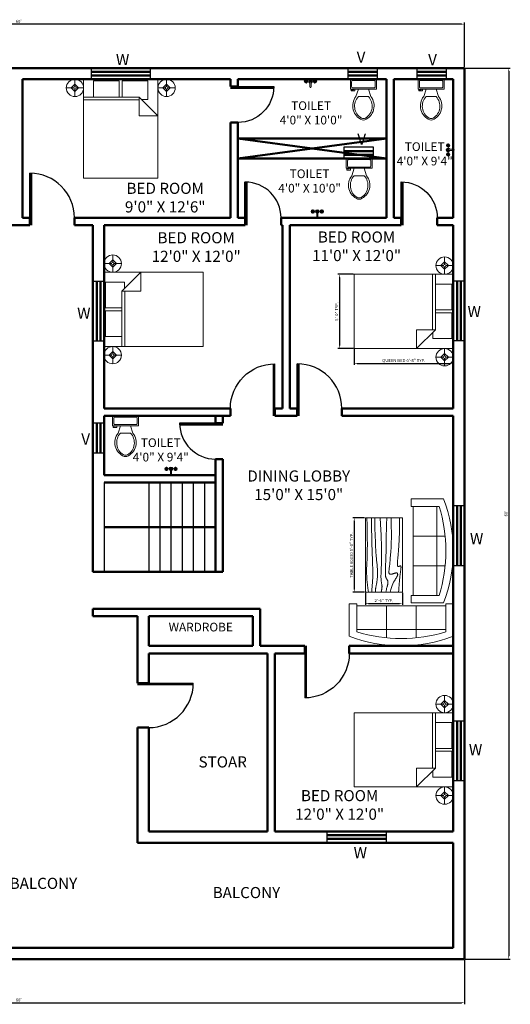
# Model space of a CAD drawing. Units: inches. Extents: x 2663 to 4539, y 2314 to 3111.
# Tile 4 of 4: x 4143 to 4539, y 2316 to 3111. Entities that reach past the tile are written whole.
import ezdxf

# ---------------------------------------------------------------- set-up
doc = ezdxf.new("R2010")
doc.units = ezdxf.units.IN
for name, color, linetype, lineweight in [('A-ANNO-DIMS', 2, 'Continuous', 18), ('A-ANNO-TEXT', 7, 'Continuous', 18), ('A-AREA-IDEN', 3, 'Continuous', 25), ('A-DOOR', 4, 'Continuous', 25), ('A-FLOR-FIXT', 8, 'Continuous', 18), ('A-FLOR-STRS', 2, 'Continuous', 25), ('A-FURN', 8, 'Continuous', 18), ('A-GLAZ', 3, 'Continuous', 25), ('A-WALL', 7, 'Continuous', 50)]:
    doc.layers.add(name, color=color, linetype=linetype, lineweight=lineweight)
doc.styles.get("Standard").update_dxf_attribs({"font": 'arial.ttf'})
doc.dimstyles.new('ISO-25', dxfattribs={"dimtxt": 2.5, "dimasz": 2.5, "dimexe": 1.25, "dimexo": 0.625, "dimtad": 1, "dimdec": 0, "dimlunit": 3, "dimtxsty": 'Standard', "dimcen": 2.5, "dimadec": 0, "dimazin": 0, "dimtfac": 1, "dimtdec": 0, "dimtmove": 0, "dimatfit": 3, "dimfxl": 1, "dimarcsym": 0})

# ---------------------------------------------------------------- blocks, each defined once
blk = doc.blocks.new('Toilet - top')
for p, q in [((9.5, -6), (9.5, -2)), ((-10, -8.5), (-8, -8.5)), ((-10, -9.5), (-10, -8.5)), ((-7, -9.5), (-10, -9.5)), ((-8, -8.5), (-8, -8)), ((-7, -8), (-7, -9.5)), ((-4, -8), (-6, -14)), ((4, -14), (-4, -14)), ((4, -8), (6, -14))]:
    blk.add_line(p, q)
blk.add_lwpolyline([(10.5, -8), (10.5, 0), (-10.5, 0), (-10.5, -8)], close=True)
for points in [[(-9.5, -2), (-9.5, -6)], [(8.5, -1), (-8.5, -1)], [(-8.5, -7), (8.5, -7)]]:
    blk.add_lwpolyline(points)
for centre, radius, start, end in [((-8.62, -1.88), 0.884, 81.8699, 188.1301), ((-8.62, -6.12), 0.884, 171.8699, 278.1301), ((8.62, -1.88), 0.884, 351.8699, 98.1301), ((8.62, -6.12), 0.884, 261.8699, 8.1301), ((3.52, -21.58), 12.17, 141.46911, 247.97143), ((4.2, -21.82), 11.33, 136.36773, 238.94682), ((-3.52, -21.58), 12.17, 292.02843, 38.53071), ((-4.2, -21.82), 11.33, 301.05301, 43.63209), ((0, -27.88), 4, 245.73182, 294.26817), ((0, -29), 4, 254.86053, 285.13947)]:
    blk.add_arc(centre, radius, start, end)
blk = doc.blocks.new('Faucet - Bathroom top')
for p, q in [((-4.107, 0.125), (-4.375, 0.125)), ((-3.75, 0.4788), (-3.75, 0.75)), ((-3.5, 0.482), (-3.5, 0.75)), ((-3.1461, 0.125), (-2.875, 0.125)), ((3.143, 0.125), (2.875, 0.125)), ((3.5, 0.4788), (3.5, 0.75)), ((3.75, 0.482), (3.75, 0.75)), ((4.1039, 0.125), (4.375, 0.125)), ((-4.1039, -0.125), (-4.375, -0.125)), ((-3.75, -0.4821), (-3.75, -0.75)), ((-3.5, -0.4789), (-3.5, -0.75)), ((-3.143, -0.125), (-2.875, -0.125)), ((-0.5, -0.8639), (-0.5, -4.5)), ((0.5, -4.5), (0.5, -0.8631)), ((3.1461, -0.125), (2.875, -0.125)), ((3.5, -0.4821), (3.5, -0.75)), ((3.75, -0.4789), (3.75, -0.75)), ((4.107, -0.125), (4.375, -0.125))]:
    blk.add_line(p, q)
for centre, radius in [((-3.625, 0), 1.375), ((-4.625, 0), 0.2795), ((-3.625, 0), 0.5), ((-3.625, 1), 0.2795), ((-2.625, 0), 0.2795), ((0, 0), 0.5), ((3.625, 0), 1.375), ((2.625, 0), 0.2795), ((3.625, 0), 0.5), ((3.625, 1), 0.2795), ((4.625, 0), 0.2795), ((-3.625, -1), 0.2795), ((3.625, -1), 0.2795)]:
    blk.add_circle(centre, radius)
for centre, radius, start, end in [((-3.625, 0), 1, 105.2407, 164.2093), ((-3.625, 0), 1, 16.44125, 74.07887), ((0, 0), 1.5, 289.6514, 250.3603), ((0, 0), 1, 300.3431, 239.7554), ((3.625, 0), 1, 106.12, 164.0884), ((3.625, 0), 1, 16.23422, 73.90469), ((-3.625, 0), 1, 196.2342, 253.9047), ((-3.625, 0), 1, 286.12, 344.0884), ((0, -4.5), 0.5, 180, 0), ((3.625, 0), 1, 196.4413, 254.0789), ((3.625, 0), 1, 285.2407, 344.2093)]:
    blk.add_arc(centre, radius, start, end)
blk = doc.blocks.new('Bed - Queen')
for p, q in [((0, -80.00003), (0, 0)), ((0, 0), (59.99999, 0)), ((59.99999, 0), (59.99999, -80.00003)), ((7.99999, -1.2), (28.79998, -1.2)), ((7.99999, -14.4), (7.99999, -1.2)), ((28.79998, -1.2), (28.79998, -14.4)), ((31.19999, -1.2), (51.99999, -1.2)), ((31.19999, -14.4), (31.19999, -1.2)), ((51.99999, -1.2), (51.99999, -16.4)), ((0, -14.4), (44.8, -14.4)), ((59.99999, -29.6), (44.8, -14.4)), ((44.8, -14.4), (44.8, -29.6)), ((44.8, -16.8), (0, -16.8)), ((51.99999, -16.4), (46.79936, -16.4)), ((44.8, -29.6), (59.99999, -29.6)), ((59.99999, -80.00003), (0, -80.00003))]:
    blk.add_line(p, q)
blk = doc.blocks.new('Lamp - Table')
for p, q in [((-1, 0), (-7, 0)), ((0, 3), (-3, 0)), ((-3, 0), (0, -3)), ((0, 7), (0, 1)), ((3, 0), (0, 3)), ((0, -3), (3, 0)), ((1, 0), (7, 0)), ((0, -1), (0, -7))]:
    blk.add_line(p, q)
for radius in [7, 1]:
    blk.add_circle((0, 0), radius)
blk = doc.blocks.new('Sofa - Roundback 7 ft.')
for p, q in [((-12.00002, -32.4421), (-12.00003, -6.5971)), ((11.99997, -32.4421), (11.99998, -6.5971)), ((-36.000027, -34), (-36.000027, -11.4696)), ((-35.999844, -13.3819), (35.9998, -13.3819)), ((35.99998, -34), (35.99998, -11.4696)), ((-36.000027, -32.4421), (35.99998, -32.4421))]:
    blk.add_line(p, q)
for points in [[(-36.000027, -34), (-42.000027, -34), (-42.000027, -8)], [(41.99998, -8), (41.99998, -34), (35.99998, -34)]]:
    blk.add_lwpolyline(points)
for centre, radius, start, end in [((0, -114.25), 114.25, 68.43141, 111.5686), ((-0.00001, -127.1968), 121.1968, 72.72033, 107.2797)]:
    blk.add_arc(centre, radius, start, end)
blk = doc.blocks.new('Table - Rectangular Woodgrain 60 x 30 in.')
for p, q in [((0, 0), (0, -30)), ((60, 0), (0, 0)), ((60, -30), (60, 0)), ((0, -30), (60, -30))]:
    blk.add_line(p, q)
for points in [[(0, -2.4), (4.8155, -2.418), (9.0302, -2.4688), (12.709, -2.5477), (15.9167, -2.65), (18.7181, -2.7711), (21.1781, -2.9063), (23.3616, -3.0508), (25.3333, -3.2), (27.1477, -3.3495), (28.8172, -3.4958), (30.3437, -3.636), (31.7291, -3.7667), (32.9756, -3.8849), (34.0849, -3.9875), (35.059, -4.0714), (35.9, -4.1334), (36.6114, -4.1711), (37.2041, -4.1854), (37.6906, -4.1779), (38.0833, -4.15), (38.3948, -4.1034), (38.6375, -4.0396), (38.8239, -3.9602), (38.9666, -3.8667), (39.0764, -3.7608), (39.1573, -3.6448), (39.2116, -3.521), (39.2416, -3.3917), (39.2498, -3.2593), (39.2385, -3.1261), (39.21, -2.9944), (39.1666, -2.8667), (39.111, -2.7447), (39.0468, -2.6281), (38.978, -2.5163), (38.9083, -2.4083), (38.8418, -2.3035), (38.7823, -2.201), (38.7337, -2.1001), (38.7, -2), (38.6844, -1.9003), (38.6875, -1.8021), (38.7094, -1.707), (38.75, -1.6167), (38.8094, -1.5326), (38.8875, -1.4563), (38.9844, -1.3893), (39.1, -1.3333), (39.2351, -1.2896), (39.3937, -1.2583), (39.5804, -1.2396), (39.8, -1.2333), (40.057, -1.2396), (40.3562, -1.2583), (40.7023, -1.2896), (41.1, -1.3333), (41.5547, -1.3895), (42.0755, -1.4573), (42.6721, -1.5361), (43.3542, -1.625), (44.1316, -1.7233), (45.014, -1.8302), (46.0114, -1.9449), (47.1333, -2.0667), (48.3862, -2.1947), (49.7625, -2.3281), (51.2513, -2.4663), (52.8416, -2.6083), (54.5226, -2.7535), (56.2833, -2.9011), (58.1127, -3.0501), (60, -3.2)], [(0, -9.2), (6.5759, -9.0858), (11.9385, -9.0365), (16.2527, -9.0418), (19.6833, -9.0917), (22.3952, -9.1759), (24.5531, -9.2844), (26.322, -9.4069), (27.8666, -9.5333), (29.3241, -9.6553), (30.7203, -9.7719), (32.0532, -9.8837), (33.3208, -9.9917), (34.5213, -10.0965), (35.6526, -10.199), (36.7128, -10.2999), (37.7, -10.4), (38.6129, -10.4996), (39.4531, -10.5969), (40.223, -10.6895), (40.925, -10.775), (41.5613, -10.8512), (42.1344, -10.9156), (42.6465, -10.966), (43.1, -11), (43.4976, -11.0158), (43.8437, -11.0136), (44.143, -10.9942), (44.4, -10.9583), (44.6195, -10.9069), (44.8062, -10.8406), (44.9648, -10.7603), (45.1, -10.6667), (45.2155, -10.5598), (45.3114, -10.4365), (45.3871, -10.2929), (45.4416, -10.125), (45.4743, -9.929), (45.4844, -9.7011), (45.4709, -9.4371), (45.4333, -9.1333), (45.3716, -8.7883), (45.2896, -8.4104), (45.1919, -8.0107), (45.0833, -7.6), (44.9685, -7.1893), (44.8521, -6.7896), (44.7388, -6.4117), (44.6333, -6.0667), (44.54, -5.7628), (44.4614, -5.4979), (44.4001, -5.2675), (44.3583, -5.0667), (44.3384, -4.8909), (44.3427, -4.7354), (44.3736, -4.5956), (44.4333, -4.4667), (44.5236, -4.3453), (44.6427, -4.2333), (44.7884, -4.1339), (44.9583, -4.05), (45.1501, -3.9849), (45.3614, -3.9417), (45.59, -3.9234), (45.8333, -3.9333), (46.0915, -3.9749), (46.3734, -4.0531), (46.6906, -4.1736), (47.0542, -4.3417), (47.4756, -4.5629), (47.9661, -4.8427), (48.5372, -5.1866), (49.2, -5.6), (49.9676, -6.0844), (50.8594, -6.625), (51.8965, -7.2031), (53.1, -7.8), (54.491, -8.3969), (56.0906, -8.975), (57.9199, -9.5156), (60, -10)], [(0, -12.8), (5.1847, -12.9322), (9.6213, -13.0323), (13.3963, -13.1059), (16.5958, -13.1583), (19.3063, -13.1952), (21.614, -13.2219), (23.6054, -13.2439), (25.3666, -13.2667), (26.9728, -13.2947), (28.4531, -13.3281), (29.8256, -13.3663), (31.1083, -13.4083), (32.3191, -13.4535), (33.476, -13.501), (34.597, -13.5501), (35.7, -13.6), (36.7984, -13.6497), (37.8875, -13.6979), (38.9578, -13.743), (40, -13.7833), (41.0047, -13.8174), (41.9625, -13.8438), (42.864, -13.8607), (43.7, -13.8667), (44.4631, -13.8604), (45.1552, -13.8417), (45.7801, -13.8104), (46.3416, -13.7667), (46.8439, -13.7104), (47.2906, -13.6417), (47.6858, -13.5604), (48.0333, -13.4667), (48.3375, -13.3608), (48.6042, -13.2448), (48.8396, -13.121), (49.05, -12.9917), (49.2417, -12.8593), (49.4208, -12.7261), (49.5937, -12.5944), (49.7667, -12.4667), (49.9452, -12.3451), (50.1323, -12.2313), (50.3303, -12.1268), (50.5416, -12.0333), (50.7686, -11.9524), (51.0135, -11.8854), (51.2788, -11.8341), (51.5666, -11.8), (51.8785, -11.7843), (52.2116, -11.7865), (52.562, -11.8059), (52.926, -11.8417), (53.2998, -11.8931), (53.6795, -11.9594), (54.0614, -12.0397), (54.4416, -12.1333), (54.8223, -12.2401), (55.2293, -12.3625), (55.6942, -12.5037), (56.2489, -12.6667), (56.9251, -12.8547), (57.7545, -13.0708), (58.7689, -13.3182), (60, -13.6)], [(0, -18), (5.124, -17.7273), (9.6609, -17.5057), (13.6705, -17.3303), (17.2125, -17.1958), (20.3467, -17.0973), (23.1328, -17.0297), (25.6307, -16.9878), (27.9, -16.9667), (29.9928, -16.9617), (31.9302, -16.9703), (33.7254, -16.9907), (35.3917, -17.0208), (36.9423, -17.0588), (38.3906, -17.1026), (39.7499, -17.1503), (41.0333, -17.2), (42.2519, -17.2496), (43.4073, -17.2969), (44.4986, -17.3395), (45.525, -17.375), (46.4858, -17.4012), (47.3802, -17.4156), (48.2074, -17.416), (48.9667, -17.4), (49.6583, -17.3662), (50.2872, -17.3167), (50.8595, -17.2547), (51.3812, -17.1833), (51.8584, -17.1057), (52.2971, -17.025), (52.7034, -16.9443), (53.0833, -16.8667), (53.443, -16.7951), (53.789, -16.7313), (54.128, -16.6768), (54.4666, -16.6334), (54.8115, -16.6024), (55.1693, -16.5854), (55.5465, -16.5841), (55.95, -16.6), (56.3828, -16.6337), (56.8346, -16.6823), (57.2915, -16.7418), (57.7396, -16.8084), (58.165, -16.878), (58.5539, -16.9469), (58.8924, -17.0111), (59.1666, -17.0667), (59.3679, -17.1107), (59.5078, -17.1438), (59.6032, -17.1675), (59.6708, -17.1833), (59.7275, -17.193), (59.7901, -17.1979), (59.8753, -17.1998), (60, -17.2)], [(0, -22.4), (8.0098, -22.2501), (14.4094, -22.1011), (19.4168, -21.9535), (23.25, -21.8083), (26.1269, -21.6663), (28.2656, -21.5281), (29.884, -21.3947), (31.2, -21.2667), (32.3967, -21.1448), (33.5172, -21.0292), (34.5697, -20.9198), (35.5625, -20.8167), (36.5037, -20.7198), (37.4015, -20.6292), (38.2642, -20.5448), (39.1, -20.4667), (39.9164, -20.3951), (40.7187, -20.3313), (41.5117, -20.2768), (42.3, -20.2333), (43.0883, -20.2024), (43.8812, -20.1854), (44.6836, -20.1841), (45.5, -20.2), (46.3328, -20.234), (47.1747, -20.2844), (48.0163, -20.3488), (48.8479, -20.425), (49.66, -20.5106), (50.4429, -20.6031), (51.1872, -20.7004), (51.8833, -20.8), (52.5246, -20.8999), (53.1166, -20.9995), (53.6681, -21.0983), (54.1875, -21.1958), (54.6834, -21.2919), (55.1646, -21.3859), (55.6394, -21.4777), (56.1167, -21.5667), (56.6028, -21.6515), (57.0961, -21.7266), (57.5929, -21.7852), (58.0896, -21.8208), (58.5823, -21.8268), (59.0674, -21.7964), (59.5412, -21.723), (60, -21.6)], [(0, -25.2), (8.6355, -25.0504), (15.7026, -24.9031), (21.4049, -24.7606), (25.9458, -24.625), (29.529, -24.4988), (32.3578, -24.3844), (34.6359, -24.284), (36.5667, -24.2), (38.3213, -24.1341), (39.9417, -24.0854), (41.437, -24.0523), (42.8167, -24.0333), (44.0901, -24.0268), (45.2667, -24.0313), (46.3557, -24.0451), (47.3667, -24.0667), (48.309, -24.0947), (49.1928, -24.1287), (50.0284, -24.168), (50.826, -24.2125), (51.5959, -24.2617), (52.3483, -24.3151), (53.0935, -24.3725), (53.8417, -24.4334), (54.6009, -24.497), (55.3699, -24.561), (56.1454, -24.6226), (56.9239, -24.6792), (57.7021, -24.7279), (58.4764, -24.7662), (59.2435, -24.7911), (60, -24.8)], [(0, -28.8), (5.6867, -28.6681), (10.45, -28.5698), (14.407, -28.5012), (17.675, -28.4584), (20.3711, -28.4374), (22.6125, -28.4344), (24.5164, -28.4455), (26.2, -28.4667), (27.762, -28.4947), (29.2276, -28.5281), (30.6033, -28.5663), (31.8958, -28.6084), (33.1118, -28.6535), (34.2578, -28.7011), (35.3405, -28.7501), (36.3666, -28.8), (37.3443, -28.8497), (38.288, -28.8974), (39.2137, -28.9412), (40.1375, -28.9792), (41.0753, -29.0093), (42.0432, -29.0297), (43.0572, -29.0384), (44.1333, -29.0333), (45.2936, -29.0114), (46.5843, -28.9641), (48.0579, -28.8816), (49.7666, -28.7542), (51.7629, -28.5721), (54.0989, -28.3255), (56.8272, -28.0048), (60, -27.6)]]:
    blk.add_lwpolyline(points)
blk = doc.blocks.new('*D14')
at = {"layer": 'A-ANNO-DIMS', "color": 0, "lineweight": -2, "transparency": 16777216}
for p, q in [((3781.84, 3072.75), (3781.84, 3108.85)), ((4499.34, 3107.6), (3784.34, 3107.6)), ((4501.84, 3072.75), (4501.84, 3108.85))]:
    blk.add_line(p, q, dxfattribs=at)
at = {"layer": 'A-ANNO-DIMS', "color": 0, "transparency": 16777216}
for points in [[(3784.34, 3108.02), (3784.34, 3107.19), (3781.84, 3107.6)], [(4499.34, 3108.02), (4499.34, 3107.19), (4501.84, 3107.6)]]:
    blk.add_solid(points, dxfattribs=at)
at = {"layer": 'Defpoints', "color": 0, "transparency": 16777216}
for p in [(3781.84, 3107.6), (3781.84, 3072.12), (4501.84, 3072.12)]:
    blk.add_point(p, dxfattribs=at)
at = {"layer": 'A-ANNO-DIMS', "color": 0, "transparency": 16777216, "insert": (4141.84, 3109.51), "char_height": 2.5, "attachment_point": 5}
blk.add_mtext("60'", dxfattribs=at)
blk = doc.blocks.new('*D15')
at = {"layer": 'A-ANNO-DIMS', "color": 0, "lineweight": -2, "transparency": 16777216}
for p, q in [((4502.46, 3072.12), (4538.88, 3072.12)), ((4537.63, 3069.62), (4537.63, 2354.62)), ((4502.46, 2352.12), (4538.88, 2352.12))]:
    blk.add_line(p, q, dxfattribs=at)
at = {"layer": 'A-ANNO-DIMS', "color": 0, "transparency": 16777216}
for points in [[(4537.21, 3069.62), (4538.04, 3069.62), (4537.63, 3072.12)], [(4537.21, 2354.62), (4538.04, 2354.62), (4537.63, 2352.12)]]:
    blk.add_solid(points, dxfattribs=at)
at = {"layer": 'Defpoints', "color": 0, "transparency": 16777216}
for p in [(4501.84, 3072.12), (4501.84, 2352.12), (4537.63, 2352.12)]:
    blk.add_point(p, dxfattribs=at)
at = {"layer": 'A-ANNO-DIMS', "color": 0, "transparency": 16777216, "insert": (4535.72, 2712.12), "char_height": 2.5, "attachment_point": 5, "rotation": 90}
blk.add_mtext("60'", dxfattribs=at)
blk = doc.blocks.new('*D17')
at = {"layer": 'A-ANNO-DIMS', "color": 0, "lineweight": -2, "transparency": 16777216}
for p, q in [((3781.84, 2352.78), (3781.84, 2315.51)), ((4501.84, 2351.5), (4501.84, 2315.51)), ((3784.34, 2316.76), (4499.34, 2316.76))]:
    blk.add_line(p, q, dxfattribs=at)
at = {"layer": 'A-ANNO-DIMS', "color": 0, "transparency": 16777216}
for points in [[(3784.34, 2317.18), (3784.34, 2316.35), (3781.84, 2316.76)], [(4499.34, 2317.18), (4499.34, 2316.35), (4501.84, 2316.76)]]:
    blk.add_solid(points, dxfattribs=at)
at = {"layer": 'Defpoints', "color": 0, "transparency": 16777216}
for p in [(3781.84, 2353.4), (4501.84, 2352.12), (4501.84, 2316.76)]:
    blk.add_point(p, dxfattribs=at)
at = {"layer": 'A-ANNO-DIMS', "color": 0, "transparency": 16777216, "insert": (4141.84, 2318.67), "char_height": 2.5, "attachment_point": 5}
blk.add_mtext("60'", dxfattribs=at)
blk = doc.blocks.new('WIN-1200')
for p, q in [((0, 48), (0, 0)), ((9, 48), (0, 48)), ((0, 48), (0, 48)), ((9, 0), (9, 48)), ((0, 0), (9, 0))]:
    blk.add_line(p, q)
blk = doc.blocks.new('VENT-600')
for p, q in [((24, 9), (0, 9)), ((0, 9), (0, 0)), ((24, 0), (24, 9)), ((0, 0), (24, 0))]:
    blk.add_line(p, q)
blk = doc.blocks.new('DOOR-750')
blk.add_line((2901.63, 3055.91), (2872.63, 3055.91))
blk.add_arc((2901.63, 3055.91), 29, 180, 270)
blk = doc.blocks.new('DOOR-900')
blk.add_line((3071.63, 2949.91), (3071.63, 2985.91))
blk.add_arc((3071.63, 2949.91), 36, 0, 90)
blk = doc.blocks.new('*D36')
at = {"layer": 'A-ANNO-DIMS', "color": 0, "lineweight": -2, "transparency": 16777216}
for p, q in [((4412.84, 2844.84), (4412.84, 2832.22)), ((4492.84, 2844.84), (4492.84, 2832.22)), ((4415.34, 2833.47), (4490.34, 2833.47))]:
    blk.add_line(p, q, dxfattribs=at)
at = {"layer": 'A-ANNO-DIMS', "color": 0, "transparency": 16777216}
for points in [[(4415.34, 2833.88), (4415.34, 2833.05), (4412.84, 2833.47)], [(4490.34, 2833.88), (4490.34, 2833.05), (4492.84, 2833.47)]]:
    blk.add_solid(points, dxfattribs=at)
at = {"layer": 'Defpoints', "color": 0, "transparency": 16777216}
for p in [(4412.84, 2845.47), (4492.84, 2845.47), (4492.84, 2833.47)]:
    blk.add_point(p, dxfattribs=at)
at = {"layer": 'A-ANNO-DIMS', "color": 0, "transparency": 16777216, "insert": (4452.84, 2835.46), "char_height": 2.5, "attachment_point": 5}
blk.add_mtext('QUEEN BED 6\'-8" TYP.', dxfattribs=at)
blk = doc.blocks.new('*D37')
at = {"layer": 'A-ANNO-DIMS', "color": 0, "lineweight": -2, "transparency": 16777216}
for p, q in [((4412.21, 2905.47), (4399.59, 2905.47)), ((4400.84, 2902.97), (4400.84, 2847.97)), ((4412.21, 2845.47), (4399.59, 2845.47))]:
    blk.add_line(p, q, dxfattribs=at)
at = {"layer": 'A-ANNO-DIMS', "color": 0, "transparency": 16777216}
for points in [[(4400.42, 2902.97), (4401.26, 2902.97), (4400.84, 2905.47)], [(4400.42, 2847.97), (4401.26, 2847.97), (4400.84, 2845.47)]]:
    blk.add_solid(points, dxfattribs=at)
at = {"layer": 'Defpoints', "color": 0, "transparency": 16777216}
for p in [(4412.84, 2905.47), (4400.84, 2845.47), (4412.84, 2845.47)]:
    blk.add_point(p, dxfattribs=at)
at = {"layer": 'A-ANNO-DIMS', "color": 0, "transparency": 16777216, "insert": (4398.94, 2875.47), "char_height": 2.5, "attachment_point": 5, "rotation": 90}
blk.add_mtext('5\'-0" TYP.', dxfattribs=at)
blk = doc.blocks.new('*D40')
at = {"layer": 'A-ANNO-DIMS', "color": 0, "lineweight": -2, "transparency": 16777216}
for p, q in [((4421.23, 2708.54), (4411.61, 2708.54)), ((4412.86, 2706.04), (4412.86, 2651.04)), ((4421.23, 2648.54), (4411.61, 2648.54))]:
    blk.add_line(p, q, dxfattribs=at)
at = {"layer": 'A-ANNO-DIMS', "color": 0, "transparency": 16777216}
for points in [[(4412.44, 2706.04), (4413.27, 2706.04), (4412.86, 2708.54)], [(4412.44, 2651.04), (4413.27, 2651.04), (4412.86, 2648.54)]]:
    blk.add_solid(points, dxfattribs=at)
at = {"layer": 'Defpoints', "color": 0, "transparency": 16777216}
for p in [(4421.86, 2708.54), (4412.86, 2648.54), (4421.86, 2648.54)]:
    blk.add_point(p, dxfattribs=at)
at = {"layer": 'A-ANNO-DIMS', "color": 0, "transparency": 16777216, "insert": (4410.95, 2678.54), "char_height": 2.5, "attachment_point": 5, "rotation": 90}
blk.add_mtext('TABLE 60X30 5\'-0" TYP.', dxfattribs=at)
blk = doc.blocks.new('*D41')
at = {"layer": 'A-ANNO-DIMS', "color": 0, "lineweight": -2, "transparency": 16777216}
for p, q in [((4421.86, 2647.92), (4421.86, 2638.29)), ((4451.86, 2647.92), (4451.86, 2638.29)), ((4424.36, 2639.54), (4449.36, 2639.54))]:
    blk.add_line(p, q, dxfattribs=at)
at = {"layer": 'A-ANNO-DIMS', "color": 0, "transparency": 16777216}
for points in [[(4424.36, 2639.96), (4424.36, 2639.13), (4421.86, 2639.54)], [(4449.36, 2639.96), (4449.36, 2639.13), (4451.86, 2639.54)]]:
    blk.add_solid(points, dxfattribs=at)
at = {"layer": 'Defpoints', "color": 0, "transparency": 16777216}
for p in [(4421.86, 2648.54), (4451.86, 2648.54), (4451.86, 2639.54)]:
    blk.add_point(p, dxfattribs=at)
at = {"layer": 'A-ANNO-DIMS', "color": 0, "transparency": 16777216, "insert": (4436.86, 2641.44), "char_height": 2.5, "attachment_point": 5}
blk.add_mtext('2\'-6" TYP.', dxfattribs=at)

msp = doc.modelspace()

# ---------------------------------------------------------------- linework, layer by layer
at = {"layer": 'A-DOOR'}
msp.add_arc((4324.84, 2951.12), 28.87, 0, 90, dxfattribs=at)
at = {"layer": 'A-FLOR-STRS'}
for p, q in [((4210.84, 2737.12), (4210.84, 2665.12)), ((4246.84, 2737.12), (4246.84, 2665.12)), ((4255.84, 2737.12), (4255.84, 2665.12)), ((4264.84, 2737.12), (4264.84, 2665.12)), ((4273.84, 2737.12), (4273.84, 2665.12)), ((4282.84, 2737.12), (4282.84, 2665.12)), ((4291.84, 2737.12), (4291.84, 2665.12))]:
    msp.add_line(p, q, dxfattribs=at)
at = {"layer": 'A-WALL'}
for p, q in [((3781.84, 3072.12), (4501.84, 3072.12)), ((4501.84, 3072.12), (4501.84, 2352.12)), ((4248.28, 3069.12), (4200.28, 3069.12)), ((4200.28, 3066.12), (4248.28, 3066.12)), ((4431.65, 3069.12), (4407.65, 3069.12)), ((4407.65, 3066.12), (4431.65, 3066.12)), ((4487.4, 3069.12), (4463.4, 3069.12)), ((4463.4, 3066.12), (4487.4, 3066.12)), ((4144.84, 3063.12), (4144.84, 2951.12)), ((4144.84, 3063.12), (4312.84, 3063.12)), ((4312.84, 3063.12), (4312.84, 3057.12)), ((4312.84, 3063.12), (4312.84, 3057.12)), ((4318.84, 3057.12), (4312.84, 3057.12)), ((4318.84, 3056.12), (4312.84, 3056.12)), ((4318.84, 3063.12), (4318.84, 3057.12)), ((4318.84, 3063.12), (4438.84, 3063.12)), ((4318.84, 3063.12), (4318.84, 3057.12)), ((4318.84, 3056.12), (4347.84, 3056.12)), ((4438.84, 3063.12), (4438.84, 2951.12)), ((4444.84, 3063.12), (4444.84, 2951.12)), ((4444.84, 3063.12), (4492.84, 3063.12)), ((4492.84, 3063.12), (4492.84, 2951.12)), ((4312.84, 3028.12), (4318.84, 3028.12)), ((4312.84, 3028.12), (4312.84, 2951.12)), ((4312.84, 3028.12), (4312.84, 2951.12)), ((4318.84, 3028.12), (4318.84, 2951.12)), ((4318.84, 3015.12), (4438.84, 3015.12)), ((4438.84, 3015.12), (4318.84, 2999.12)), ((4318.84, 2999.12), (4318.84, 3015.12)), ((4318.84, 3015.12), (4438.84, 2999.12)), ((4428.5, 3005.09), (4404.5, 3005.09)), ((4404.5, 3002.09), (4428.5, 3002.09)), ((4318.84, 2999.12), (4438.84, 2999.12)), ((4151.84, 2951.12), (4151.84, 2987.12)), ((4324.84, 2951.12), (4324.84, 2980.12)), ((4325.84, 2951.12), (4325.84, 2980.12)), ((4451.84, 2951.12), (4451.84, 2980.12)), ((4132.84, 2945.12), (4150.84, 2945.12)), ((4144.84, 2951.12), (4150.84, 2951.12)), ((4144.84, 2951.12), (4150.84, 2951.12)), ((4150.84, 2951.12), (4150.84, 2945.12)), ((4151.84, 2951.12), (4151.84, 2945.12)), ((4186.84, 2945.12), (4186.84, 2951.12)), ((4186.84, 2951.12), (4312.84, 2951.12)), ((4186.84, 2945.12), (4201.84, 2945.12)), ((4201.84, 2945.12), (4201.84, 2791.12)), ((4210.84, 2945.12), (4210.84, 2797.12)), ((4210.84, 2945.12), (4324.84, 2945.12)), ((4318.84, 2951.12), (4324.84, 2951.12)), ((4318.84, 2951.12), (4324.84, 2951.12)), ((4324.84, 2951.12), (4324.84, 2945.12)), ((4325.84, 2951.12), (4325.84, 2945.12)), ((4353.71, 2945.12), (4353.71, 2951.12)), ((4353.71, 2951.12), (4438.84, 2951.12)), ((4353.71, 2945.12), (4354.84, 2945.12)), ((4354.84, 2945.12), (4353.71, 2945.12)), ((4353.71, 2945.12), (4354.84, 2945.12)), ((4354.84, 2945.12), (4354.84, 2797.12)), ((4360.84, 2945.12), (4360.84, 2797.12)), ((4360.84, 2945.12), (4360.84, 2797.12)), ((4360.84, 2945.12), (4450.84, 2945.12)), ((4444.84, 2951.12), (4450.84, 2951.12)), ((4444.84, 2951.12), (4450.84, 2951.12)), ((4450.84, 2951.12), (4450.84, 2945.12)), ((4451.84, 2951.12), (4451.84, 2945.12)), ((4479.84, 2945.12), (4479.84, 2951.12)), ((4479.84, 2951.12), (4492.84, 2951.12)), ((4479.84, 2945.12), (4492.84, 2945.12)), ((4492.84, 2945.12), (4492.84, 2797.12)), ((4204.84, 2899.67), (4204.84, 2851.67)), ((4207.84, 2851.67), (4207.84, 2899.67)), ((4495.84, 2900.01), (4495.84, 2852.01)), ((4498.84, 2852.01), (4498.84, 2900.01)), ((4347.84, 2797.12), (4347.84, 2833.12)), ((4367.84, 2797.12), (4367.84, 2833.12)), ((4210.84, 2797.12), (4312.84, 2797.12)), ((4312.84, 2791.12), (4312.84, 2797.12)), ((4347.84, 2797.12), (4347.84, 2791.12)), ((4354.84, 2797.12), (4348.84, 2797.12)), ((4348.84, 2797.12), (4348.84, 2791.12)), ((4348.84, 2797.12), (4354.84, 2797.12)), ((4360.84, 2797.12), (4366.84, 2797.12)), ((4360.84, 2797.12), (4366.84, 2797.12)), ((4366.84, 2797.12), (4366.84, 2791.12)), ((4367.84, 2797.12), (4367.84, 2791.12)), ((4402.84, 2791.12), (4402.84, 2797.12)), ((4402.84, 2797.12), (4492.84, 2797.12)), ((4201.84, 2791.12), (4201.84, 2746.12)), ((4204.84, 2785.25), (4204.84, 2761.25)), ((4207.84, 2761.25), (4207.84, 2785.25)), ((4210.84, 2791.12), (4312.84, 2791.12)), ((4210.84, 2791.12), (4210.84, 2743.12)), ((4300.84, 2791.12), (4300.84, 2785.12)), ((4300.84, 2791.12), (4300.84, 2785.12)), ((4300.84, 2791.12), (4300.84, 2785.12)), ((4300.84, 2785.12), (4306.84, 2785.12)), ((4306.84, 2791.12), (4306.84, 2785.12)), ((4306.84, 2791.12), (4306.84, 2785.12)), ((4348.84, 2791.12), (4366.84, 2791.12)), ((4402.84, 2791.12), (4492.84, 2791.12)), ((4492.84, 2791.12), (4492.84, 2635.12)), ((4300.84, 2784.12), (4271.84, 2784.12)), ((4300.84, 2784.12), (4306.84, 2784.12)), ((4306.84, 2756.12), (4300.84, 2756.12)), ((4300.84, 2756.12), (4300.84, 2737.12)), ((4300.84, 2756.12), (4300.84, 2665.12)), ((4306.84, 2756.12), (4306.84, 2737.12)), ((4306.84, 2756.12), (4306.84, 2665.12)), ((4201.84, 2746.12), (4201.84, 2665.12)), ((4210.84, 2743.12), (4300.84, 2743.12)), ((4210.84, 2737.12), (4300.84, 2737.12)), ((4495.84, 2718.26), (4495.84, 2670.26)), ((4498.84, 2670.26), (4498.84, 2718.26)), ((4210.84, 2701.12), (4300.84, 2701.12)), ((4201.84, 2665.12), (4210.84, 2665.12)), ((4210.84, 2665.12), (4300.84, 2665.12)), ((4300.84, 2665.12), (4306.84, 2665.12)), ((4201.84, 2635.12), (4237.84, 2635.12)), ((4201.84, 2635.12), (4201.84, 2629.12)), ((4210.84, 2635.12), (4336.84, 2635.12)), ((4336.84, 2629.12), (4336.84, 2635.12)), ((4492.84, 2605.12), (4492.84, 2635.12)), ((4201.84, 2629.12), (4204.84, 2629.12)), ((4204.84, 2629.12), (4237.84, 2629.12)), ((4237.84, 2629.12), (4237.84, 2575.12)), ((4246.84, 2629.12), (4246.84, 2605.12)), ((4246.84, 2629.12), (4330.84, 2629.12)), ((4330.84, 2629.12), (4330.84, 2605.12)), ((4336.84, 2629.12), (4336.84, 2605.12)), ((4492.84, 2629.12), (4492.84, 2455.12)), ((4246.84, 2605.12), (4330.84, 2605.12)), ((4336.84, 2605.12), (4372.84, 2605.12)), ((4372.84, 2599.12), (4372.84, 2605.12)), ((4373.84, 2599.12), (4373.84, 2605.12)), ((4408.84, 2605.12), (4408.84, 2599.12)), ((4408.84, 2605.12), (4492.84, 2605.12)), ((4246.84, 2599.12), (4336.84, 2599.12)), ((4246.84, 2599.12), (4246.84, 2575.12)), ((4246.84, 2599.12), (4246.84, 2575.12)), ((4336.84, 2599.12), (4342.84, 2599.12)), ((4342.84, 2599.12), (4342.84, 2455.12)), ((4348.84, 2599.12), (4348.84, 2455.12)), ((4348.84, 2599.12), (4372.84, 2599.12)), ((4348.84, 2599.12), (4372.84, 2599.12)), ((4373.84, 2599.12), (4373.84, 2563.12)), ((4408.84, 2599.12), (4492.84, 2599.12)), ((4246.84, 2575.12), (4237.84, 2575.12)), ((4246.84, 2574.12), (4237.84, 2574.12)), ((4246.84, 2574.12), (4282.84, 2574.12)), ((4237.84, 2539.12), (4246.84, 2539.12)), ((4237.84, 2539.12), (4237.84, 2446.12)), ((4246.84, 2539.12), (4246.84, 2455.12)), ((4495.84, 2544.36), (4495.84, 2496.36)), ((4498.84, 2496.36), (4498.84, 2544.36)), ((4246.84, 2455.12), (4336.84, 2455.12)), ((4336.84, 2455.12), (4342.84, 2455.12)), ((4348.84, 2455.12), (4492.84, 2455.12)), ((4438.84, 2452.12), (4390.84, 2452.12)), ((4237.84, 2446.12), (4246.84, 2446.12)), ((4246.84, 2446.12), (4336.84, 2446.12)), ((4336.84, 2446.12), (4492.84, 2446.12)), ((4390.84, 2449.12), (4438.84, 2449.12)), ((4492.84, 2446.12), (4492.84, 2361.12)), ((4237.84, 2361.12), (3790.84, 2361.12)), ((4246.84, 2361.12), (4237.84, 2361.12)), ((4492.84, 2361.12), (4246.84, 2361.12)), ((4501.84, 2352.12), (3781.84, 2352.12))]:
    msp.add_line(p, q, dxfattribs=at)

# ---------------------------------------------------------------- block references
at = {"layer": 'A-DOOR', "extrusion": (0, 0, -1), "zscale": -1}
for name, p in [('DOOR-750', (-7220.47, 1.21)), ('DOOR-900', (-7420.47, -152.79))]:
    msp.add_blockref(name, p, dxfattribs=at)
at = {"layer": 'A-DOOR'}
for name, p in [('DOOR-900', (1079.21, 1.21)), ('DOOR-900', (1295.21, -152.79)), ('DOOR-750', (1399.21, -270.79))]:
    msp.add_blockref(name, p, dxfattribs=at)
at = {"layer": 'A-DOOR', "extrusion": (0, 0, -1), "zscale": -1}
for name, p, rotation in [('DOOR-750', (-7506.75, 5852.76), 270.0000000000005), ('DOOR-900', (-1301.21, 5549.04), 180)]:
    msp.add_blockref(name, p, dxfattribs=dict(at, rotation=rotation))
at = {"layer": 'A-DOOR', "rotation": 269.9999999999989}
msp.add_blockref('DOOR-900', (1296.92, 5646.76), dxfattribs=at)
at = {"layer": 'A-FLOR-FIXT'}
for name, p in [('Faucet - Bathroom top', (4377.53, 3061.4)), ('Toilet - top', (4420.24, 3063.12)), ('Toilet - top', (4474.93, 3063.12)), ('Toilet - top', (4416.83, 2999.12)), ('Faucet - Bathroom top', (4383.04, 2956.18)), ('Toilet - top', (4228.13, 2791.12)), ('Faucet - Bathroom top', (4264.85, 2748.19))]:
    msp.add_blockref(name, p, dxfattribs=at)
at = {"layer": 'A-FLOR-FIXT', "rotation": 90}
msp.add_blockref('Faucet - Bathroom top', (4488.61, 3006), dxfattribs=at)
at = {"layer": 'A-FURN'}
for name, p in [('Lamp - Table', (4187.28, 3056.12)), ('Bed - Queen', (4194.28, 3063.12)), ('Lamp - Table', (4261.28, 3056.12))]:
    msp.add_blockref(name, p, dxfattribs=at)
for name, p, rotation in [('Lamp - Table', (4217.84, 2914.11), 89.99999999999953), ('Lamp - Table', (4485.84, 2912.47), 270), ('Bed - Queen', (4210.84, 2847.11), 89.99999999999953), ('Bed - Queen', (4492.84, 2905.47), 270), ('Lamp - Table', (4217.84, 2840.11), 89.99999999999953), ('Lamp - Table', (4485.84, 2838.47), 270), ('Sofa - Roundback 7 ft.', (4492.84, 2681.93), 270), ('Table - Rectangular Woodgrain 60 x 30 in.', (4451.86, 2708.54), 270), ('Sofa - Roundback 7 ft.', (4450.84, 2605.12), 180), ('Lamp - Table', (4485.84, 2558.16), 270), ('Bed - Queen', (4492.84, 2551.16), 270), ('Lamp - Table', (4485.84, 2484.16), 270)]:
    msp.add_blockref(name, p, dxfattribs=dict(at, rotation=rotation))
at = {"layer": 'A-GLAZ'}
for name, p, rotation in [('WIN-1200', (4248.28, 3063.12), 89.99999999999683), ('VENT-600', (4201.84, 2785.25), 270.0000000000007), ('WIN-1200', (4438.84, 2446.12), 89.99999999999704)]:
    msp.add_blockref(name, p, dxfattribs=dict(at, rotation=rotation))
for name, p in [('VENT-600', (4407.65, 3063.12)), ('VENT-600', (4463.4, 3063.12)), ('VENT-600', (4404.5, 2999.09)), ('WIN-1200', (4201.84, 2851.67)), ('WIN-1200', (4492.84, 2852.02)), ('WIN-1200', (4492.84, 2670.26)), ('WIN-1200', (4492.84, 2496.36))]:
    msp.add_blockref(name, p, dxfattribs=at)

# ---------------------------------------------------------------- texts
at = {"layer": 'A-ANNO-TEXT', "char_height": 9, "attachment_point": 1}
for s, insert in [('\\pxqc;W', (4175.06, 3083.47)), ('\\pxqc;V', (4367.59, 3085.46)), ('\\pxqc;V', (4425.32, 3083.42)), ('\\pxqc;V', (4368.1, 3019.11)), ('\\pxqc;W', (4143.74, 2878.49)), ('\\pxqc;W', (4459.01, 2879.89)), ('\\pxqc;V', (4145.2, 2776.83)), ('\\pxqc;W', (4460.93, 2696.35)), ('\\pxqc;W', (4460.1, 2525.77)), ('\\pxqc;W', (4367.02, 2442.55))]:
    msp.add_mtext_dynamic_manual_height_columns(s, width=101.4958, gutter_width=12.5, heights=[0], dxfattribs=dict(at, insert=insert))
at = {"layer": 'A-AREA-IDEN', "attachment_point": 1}
for s, width, insert, char_height in [('\\pxqc;TOILET^J4\'0" X 10\'0"', 66.2554, (4344.84, 3045.24), 7), ('\\pxqc;TOILET^J4\'0" X 9\'4"', 66.2554, (4436.62, 3012.12), 7), ('\\pxqc;TOILET^J4\'0" X 10\'0"', 66.2554, (4343.67, 2990.2), 7), ('\\pxqc;BED ROOM \\P9\'0" X 12\'6"', 107.0744, (4206.67, 2979.43), 9), ('\\pxqc;BED ROOM \\P12\'0" X 12\'0"', 107.0744, (4231.7, 2939.5), 9), ('\\pxqc;BED ROOM \\P11\'0" X 12\'0"', 107.0744, (4361.2, 2940.08), 9), ('\\pxqc;TOILET^J4\'0" X 9\'4"', 66.2554, (4223.45, 2772.87), 7), ('\\pxqc;DINING LOBBY\\P15\'0" X 15\'0"', 101.6643, (4317.18, 2746.96), 9), ('\\pxqc;WARDROBE', 73.6922, (4252.05, 2623.87), 7), ('\\pxqc;STOAR', 82.7658, (4265.26, 2515.89), 9), ('\\pxqc;BED ROOM \\P12\'0" X 12\'0"', 107.0744, (4347.51, 2488.64), 9), ('\\pxqc;BALCONY', 201.8325, (4060.93, 2417.75), 9), ('\\pxqc;BALCONY', 201.8325, (4224.87, 2410.3), 9)]:
    msp.add_mtext_dynamic_manual_height_columns(s, width=width, gutter_width=12.5, heights=[0], dxfattribs=dict(at, insert=insert, char_height=char_height))

# ---------------------------------------------------------------- dimensions: what is measured, and where the dimension line sits
at = {"layer": 'A-ANNO-DIMS'}
for base, p1, p2, picture, middle in [((3781.84, 3107.6), (4501.84, 3072.12), (3781.84, 3072.12), '*D14', (4141.84, 3109.51)), ((4501.84, 2316.76), (3781.84, 2353.4), (4501.84, 2352.12), '*D17', (4141.84, 2318.67))]:
    dim = msp.add_linear_dim(base=base, p1=p1, p2=p2, dimstyle='ISO-25', override={"dimclrd": 0, "dimclre": 0, "dimclrt": 0}, dxfattribs=at)
    dim.commit()
    dim.dimension.update_dxf_attribs({"geometry": picture, "text_midpoint": middle})
dim = msp.add_linear_dim(base=(4537.63, 2352.12), p1=(4501.84, 3072.12), p2=(4501.84, 2352.12), angle=90, dimstyle='ISO-25', override={"dimclrd": 0, "dimclre": 0, "dimclrt": 0}, dxfattribs=at)
dim.commit()
dim.dimension.update_dxf_attribs({"geometry": '*D15', "text_midpoint": (4535.72, 2712.12)})
for base, p1, p2, text, picture, middle in [((4400.84, 2845.47), (4412.84, 2905.47), (4412.84, 2845.47), '<> TYP.', '*D37', (4398.94, 2875.47)), ((4412.86, 2648.54), (4421.86, 2708.54), (4421.86, 2648.54), 'TABLE 60X30 <> TYP.', '*D40', (4410.95, 2678.54))]:
    dim = msp.add_linear_dim(base=base, p1=p1, p2=p2, angle=270, text=text, dimstyle='ISO-25', override={"dimdec": 1, "dimrnd": 0, "dimzin": 1, "dimlunit": 4, "dimfrac": 2}, dxfattribs=at)
    dim.commit()
    dim.dimension.update_dxf_attribs({"geometry": picture, "text_midpoint": middle})
for base, p1, p2, text, picture, middle in [((4492.84, 2833.47), (4412.84, 2845.47), (4492.84, 2845.47), 'QUEEN BED <> TYP.', '*D36', (4452.84, 2835.46)), ((4451.86, 2639.54), (4421.86, 2648.54), (4451.86, 2648.54), '<> TYP.', '*D41', (4436.86, 2641.44))]:
    dim = msp.add_linear_dim(base=base, p1=p1, p2=p2, text=text, dimstyle='ISO-25', override={"dimdec": 1, "dimrnd": 0, "dimzin": 1, "dimlunit": 4, "dimfrac": 2}, dxfattribs=at)
    dim.commit()
    dim.dimension.update_dxf_attribs({"geometry": picture, "text_midpoint": middle})

doc.saveas('drawing.dxf')
